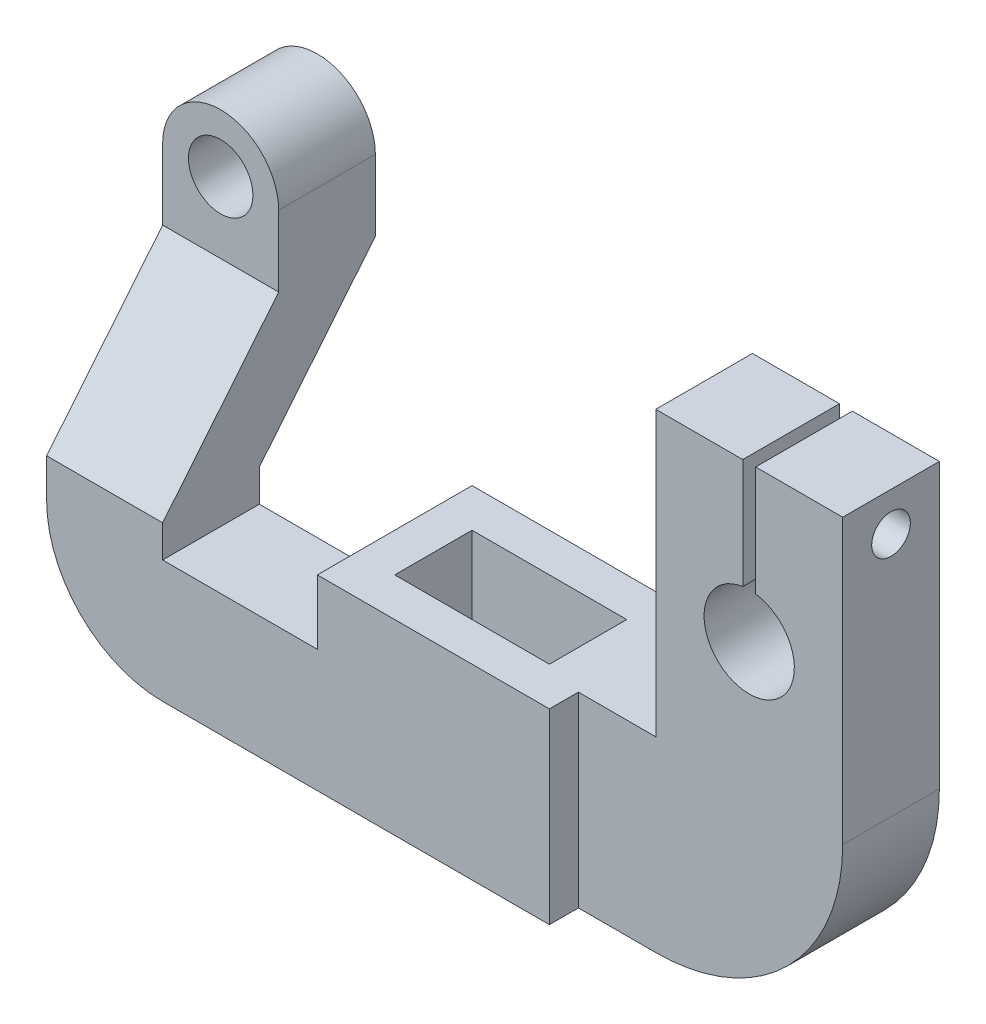
ISO-10303-21;
HEADER;
FILE_DESCRIPTION(('STEP AP214'),'2;1');
FILE_NAME('part.step','',(''),(''),'','','');
FILE_SCHEMA(('AUTOMOTIVE_DESIGN { 1 0 10303 214 1 1 1 1 }'));
ENDSEC;
DATA;
#1=APPLICATION_CONTEXT('core data for automotive mechanical design processes');
#2=APPLICATION_PROTOCOL_DEFINITION('international standard','automotive_design',2000,#1);
#3=PRODUCT_CONTEXT('',#1,'mechanical');
#4=PRODUCT('Part','Part','',(#3));
#5=PRODUCT_RELATED_PRODUCT_CATEGORY('part','',(#4));
#6=PRODUCT_DEFINITION_FORMATION('','',#4);
#7=PRODUCT_DEFINITION_CONTEXT('part definition',#1,'design');
#8=PRODUCT_DEFINITION('design','',#6,#7);
#9=PRODUCT_DEFINITION_SHAPE('','',#8);
#10=(LENGTH_UNIT() NAMED_UNIT(*) SI_UNIT(.MILLI.,.METRE.));
#11=(NAMED_UNIT(*) PLANE_ANGLE_UNIT() SI_UNIT($,.RADIAN.));
#12=(NAMED_UNIT(*) SI_UNIT($,.STERADIAN.) SOLID_ANGLE_UNIT());
#13=UNCERTAINTY_MEASURE_WITH_UNIT(LENGTH_MEASURE(1.E-05),#10,'distance_accuracy_value','');
#14=(GEOMETRIC_REPRESENTATION_CONTEXT(3) GLOBAL_UNCERTAINTY_ASSIGNED_CONTEXT((#13)) GLOBAL_UNIT_ASSIGNED_CONTEXT((#10,
#11,#12)) REPRESENTATION_CONTEXT('',''));
#15=CARTESIAN_POINT('',(0.,0.,0.));
#16=DIRECTION('',(0.,0.,1.));
#17=DIRECTION('',(1.,0.,0.));
#18=AXIS2_PLACEMENT_3D('',#15,#16,#17);
#19=CARTESIAN_POINT('',(0.,73.,-19.5));
#20=DIRECTION('',(0.,-1.,0.));
#21=DIRECTION('',(0.,0.,-1.));
#22=AXIS2_PLACEMENT_3D('',#19,#20,#21);
#23=PLANE('',#22);
#24=DIRECTION('',(1.,0.,0.));
#25=VECTOR('',#24,1.);
#26=CARTESIAN_POINT('',(0.,73.,-4.5));
#27=LINE('',#26,#25);
#28=CARTESIAN_POINT('',(72.,73.,-4.5));
#29=VERTEX_POINT('',#28);
#30=CARTESIAN_POINT('',(85.5,73.,-4.5));
#31=VERTEX_POINT('',#30);
#32=EDGE_CURVE('E374',#29,#31,#27,.T.);
#33=ORIENTED_EDGE('',*,*,#32,.T.);
#34=DIRECTION('',(0.,0.,1.));
#35=VECTOR('',#34,1.);
#36=CARTESIAN_POINT('',(85.5,73.,-19.5));
#37=LINE('',#36,#35);
#38=CARTESIAN_POINT('',(85.5,73.,-19.5));
#39=VERTEX_POINT('',#38);
#40=EDGE_CURVE('E269',#39,#31,#37,.T.);
#41=ORIENTED_EDGE('',*,*,#40,.F.);
#42=DIRECTION('',(1.,0.,0.));
#43=VECTOR('',#42,1.);
#44=CARTESIAN_POINT('',(0.,73.,-19.5));
#45=LINE('',#44,#43);
#46=CARTESIAN_POINT('',(72.,73.,-19.5));
#47=VERTEX_POINT('',#46);
#48=EDGE_CURVE('E356',#47,#39,#45,.T.);
#49=ORIENTED_EDGE('',*,*,#48,.F.);
#50=DIRECTION('',(0.,0.,1.));
#51=VECTOR('',#50,1.);
#52=CARTESIAN_POINT('',(72.,73.,-19.5));
#53=LINE('',#52,#51);
#54=EDGE_CURVE('E390',#47,#29,#53,.T.);
#55=ORIENTED_EDGE('',*,*,#54,.T.);
#56=EDGE_LOOP('',(#33,#41,#49,#55));
#57=FACE_BOUND('',#56,.T.);
#58=ADVANCED_FACE('F44',(#57),#23,.F.);
#59=CARTESIAN_POINT('',(60.,0.,-24.));
#60=DIRECTION('',(1.,0.,0.));
#61=DIRECTION('',(0.,0.,-1.));
#62=AXIS2_PLACEMENT_3D('',#59,#60,#61);
#63=PLANE('',#62);
#64=DIRECTION('',(0.,0.,1.));
#65=VECTOR('',#64,1.);
#66=CARTESIAN_POINT('',(60.,0.,-24.));
#67=LINE('',#66,#65);
#68=CARTESIAN_POINT('',(60.,0.,-4.5));
#69=VERTEX_POINT('',#68);
#70=CARTESIAN_POINT('',(60.,0.,0.));
#71=VERTEX_POINT('',#70);
#72=EDGE_CURVE('E424',#69,#71,#67,.T.);
#73=ORIENTED_EDGE('',*,*,#72,.F.);
#74=DIRECTION('',(0.,1.,0.));
#75=VECTOR('',#74,1.);
#76=CARTESIAN_POINT('',(60.,0.,-4.5));
#77=LINE('',#76,#75);
#78=CARTESIAN_POINT('',(60.,29.,-4.5));
#79=VERTEX_POINT('',#78);
#80=EDGE_CURVE('E348',#69,#79,#77,.T.);
#81=ORIENTED_EDGE('',*,*,#80,.T.);
#82=DIRECTION('',(0.,0.,1.));
#83=VECTOR('',#82,1.);
#84=CARTESIAN_POINT('',(60.,29.,-24.));
#85=LINE('',#84,#83);
#86=CARTESIAN_POINT('',(60.,29.,0.));
#87=VERTEX_POINT('',#86);
#88=EDGE_CURVE('E419',#79,#87,#85,.T.);
#89=ORIENTED_EDGE('',*,*,#88,.T.);
#90=DIRECTION('',(0.,1.,0.));
#91=VECTOR('',#90,1.);
#92=CARTESIAN_POINT('',(60.,0.,0.));
#93=LINE('',#92,#91);
#94=EDGE_CURVE('E400',#71,#87,#93,.T.);
#95=ORIENTED_EDGE('',*,*,#94,.F.);
#96=EDGE_LOOP('',(#73,#81,#89,#95));
#97=FACE_BOUND('',#96,.T.);
#98=ADVANCED_FACE('F484',(#97),#63,.T.);
#99=CARTESIAN_POINT('',(-18.,0.,-15.));
#100=DIRECTION('',(1.,0.,0.));
#101=DIRECTION('',(0.,0.,-1.));
#102=AXIS2_PLACEMENT_3D('',#99,#100,#101);
#103=PLANE('',#102);
#104=DIRECTION('',(0.,1.,0.));
#105=VECTOR('',#104,1.);
#106=CARTESIAN_POINT('',(-18.,0.,0.));
#107=LINE('',#106,#105);
#108=CARTESIAN_POINT('',(-18.,17.9999999999999,0.));
#109=VERTEX_POINT('',#108);
#110=CARTESIAN_POINT('',(-18.,24.,0.));
#111=VERTEX_POINT('',#110);
#112=EDGE_CURVE('E420',#109,#111,#107,.T.);
#113=ORIENTED_EDGE('',*,*,#112,.T.);
#114=DIRECTION('',(0.,0.773957299203321,-0.633237790257263));
#115=VECTOR('',#114,1.);
#116=CARTESIAN_POINT('',(-18.,46.,-18.));
#117=LINE('',#116,#115);
#118=CARTESIAN_POINT('',(-18.,46.,-18.));
#119=VERTEX_POINT('',#118);
#120=EDGE_CURVE('E329',#111,#119,#117,.T.);
#121=ORIENTED_EDGE('',*,*,#120,.T.);
#122=DIRECTION('',(0.,-1.,0.));
#123=VECTOR('',#122,1.);
#124=CARTESIAN_POINT('',(-18.,57.,-18.));
#125=LINE('',#124,#123);
#126=CARTESIAN_POINT('',(-18.,57.,-18.));
#127=VERTEX_POINT('',#126);
#128=EDGE_CURVE('E312',#127,#119,#125,.T.);
#129=ORIENTED_EDGE('',*,*,#128,.F.);
#130=DIRECTION('',(0.,0.,-1.));
#131=VECTOR('',#130,1.);
#132=CARTESIAN_POINT('',(-18.,57.,-18.));
#133=LINE('',#132,#131);
#134=CARTESIAN_POINT('',(-18.,57.,-33.));
#135=VERTEX_POINT('',#134);
#136=EDGE_CURVE('E318',#127,#135,#133,.T.);
#137=ORIENTED_EDGE('',*,*,#136,.T.);
#138=DIRECTION('',(0.,-1.,0.));
#139=VECTOR('',#138,1.);
#140=CARTESIAN_POINT('',(-18.,57.,-33.));
#141=LINE('',#140,#139);
#142=CARTESIAN_POINT('',(-18.,46.,-33.));
#143=VERTEX_POINT('',#142);
#144=EDGE_CURVE('E311',#135,#143,#141,.T.);
#145=ORIENTED_EDGE('',*,*,#144,.T.);
#146=DIRECTION('',(0.,-0.773957299203321,0.633237790257263));
#147=VECTOR('',#146,1.);
#148=CARTESIAN_POINT('',(-18.,46.,-33.));
#149=LINE('',#148,#147);
#150=CARTESIAN_POINT('',(-18.,24.,-15.));
#151=VERTEX_POINT('',#150);
#152=EDGE_CURVE('E331',#143,#151,#149,.T.);
#153=ORIENTED_EDGE('',*,*,#152,.T.);
#154=DIRECTION('',(0.,1.,0.));
#155=VECTOR('',#154,1.);
#156=CARTESIAN_POINT('',(-18.,0.,-15.));
#157=LINE('',#156,#155);
#158=CARTESIAN_POINT('',(-18.,17.9999999999999,-15.));
#159=VERTEX_POINT('',#158);
#160=EDGE_CURVE('E427',#159,#151,#157,.T.);
#161=ORIENTED_EDGE('',*,*,#160,.F.);
#162=DIRECTION('',(0.,0.,1.));
#163=VECTOR('',#162,1.);
#164=CARTESIAN_POINT('',(-18.,17.9999999999999,-15.));
#165=LINE('',#164,#163);
#166=EDGE_CURVE('E446',#159,#109,#165,.T.);
#167=ORIENTED_EDGE('',*,*,#166,.T.);
#168=EDGE_LOOP('',(#113,#121,#129,#137,#145,#153,#161,#167));
#169=FACE_BOUND('',#168,.T.);
#170=ADVANCED_FACE('F50',(#169),#103,.F.);
#171=CARTESIAN_POINT('',(0.,0.,-15.));
#172=DIRECTION('',(1.,0.,0.));
#173=DIRECTION('',(0.,1.,0.));
#174=AXIS2_PLACEMENT_3D('',#171,#172,#173);
#175=PLANE('',#174);
#176=DIRECTION('',(0.,1.,0.));
#177=VECTOR('',#176,1.);
#178=CARTESIAN_POINT('',(0.,0.,0.));
#179=LINE('',#178,#177);
#180=CARTESIAN_POINT('',(0.,19.,0.));
#181=VERTEX_POINT('',#180);
#182=CARTESIAN_POINT('',(0.,24.,0.));
#183=VERTEX_POINT('',#182);
#184=EDGE_CURVE('E462',#181,#183,#179,.T.);
#185=ORIENTED_EDGE('',*,*,#184,.F.);
#186=DIRECTION('',(0.,0.,1.));
#187=VECTOR('',#186,1.);
#188=CARTESIAN_POINT('',(0.,19.,-15.));
#189=LINE('',#188,#187);
#190=CARTESIAN_POINT('',(0.,19.,-15.));
#191=VERTEX_POINT('',#190);
#192=EDGE_CURVE('E11',#191,#181,#189,.T.);
#193=ORIENTED_EDGE('',*,*,#192,.F.);
#194=DIRECTION('',(0.,1.,0.));
#195=VECTOR('',#194,1.);
#196=CARTESIAN_POINT('',(0.,0.,-15.));
#197=LINE('',#196,#195);
#198=CARTESIAN_POINT('',(0.,24.,-15.));
#199=VERTEX_POINT('',#198);
#200=EDGE_CURVE('E441',#191,#199,#197,.T.);
#201=ORIENTED_EDGE('',*,*,#200,.T.);
#202=DIRECTION('',(0.,-0.773957299203321,0.633237790257263));
#203=VECTOR('',#202,1.);
#204=CARTESIAN_POINT('',(0.,46.,-33.));
#205=LINE('',#204,#203);
#206=CARTESIAN_POINT('',(0.,46.,-33.));
#207=VERTEX_POINT('',#206);
#208=EDGE_CURVE('E334',#207,#199,#205,.T.);
#209=ORIENTED_EDGE('',*,*,#208,.F.);
#210=DIRECTION('',(0.,1.,0.));
#211=VECTOR('',#210,1.);
#212=CARTESIAN_POINT('',(0.,46.,-33.));
#213=LINE('',#212,#211);
#214=CARTESIAN_POINT('',(0.,57.,-33.));
#215=VERTEX_POINT('',#214);
#216=EDGE_CURVE('E308',#207,#215,#213,.T.);
#217=ORIENTED_EDGE('',*,*,#216,.T.);
#218=DIRECTION('',(0.,0.,-1.));
#219=VECTOR('',#218,1.);
#220=CARTESIAN_POINT('',(0.,57.,-18.));
#221=LINE('',#220,#219);
#222=CARTESIAN_POINT('',(0.,57.,-18.));
#223=VERTEX_POINT('',#222);
#224=EDGE_CURVE('E330',#223,#215,#221,.T.);
#225=ORIENTED_EDGE('',*,*,#224,.F.);
#226=DIRECTION('',(0.,1.,0.));
#227=VECTOR('',#226,1.);
#228=CARTESIAN_POINT('',(0.,46.,-18.));
#229=LINE('',#228,#227);
#230=CARTESIAN_POINT('',(0.,46.,-18.));
#231=VERTEX_POINT('',#230);
#232=EDGE_CURVE('E310',#231,#223,#229,.T.);
#233=ORIENTED_EDGE('',*,*,#232,.F.);
#234=DIRECTION('',(0.,0.773957299203321,-0.633237790257263));
#235=VECTOR('',#234,1.);
#236=CARTESIAN_POINT('',(0.,46.,-18.));
#237=LINE('',#236,#235);
#238=EDGE_CURVE('E332',#183,#231,#237,.T.);
#239=ORIENTED_EDGE('',*,*,#238,.F.);
#240=EDGE_LOOP('',(#185,#193,#201,#209,#217,#225,#233,#239));
#241=FACE_BOUND('',#240,.T.);
#242=ADVANCED_FACE('F507',(#241),#175,.T.);
#243=CARTESIAN_POINT('',(0.,19.,-15.));
#244=DIRECTION('',(0.,1.,0.));
#245=DIRECTION('',(-1.,0.,0.));
#246=AXIS2_PLACEMENT_3D('',#243,#244,#245);
#247=PLANE('',#246);
#248=DIRECTION('',(-1.,0.,0.));
#249=VECTOR('',#248,1.);
#250=CARTESIAN_POINT('',(0.,19.,0.));
#251=LINE('',#250,#249);
#252=CARTESIAN_POINT('',(24.,19.,0.));
#253=VERTEX_POINT('',#252);
#254=EDGE_CURVE('E456',#253,#181,#251,.T.);
#255=ORIENTED_EDGE('',*,*,#254,.F.);
#256=DIRECTION('',(0.,0.,1.));
#257=VECTOR('',#256,1.);
#258=CARTESIAN_POINT('',(24.,19.,-15.));
#259=LINE('',#258,#257);
#260=CARTESIAN_POINT('',(24.,19.,-15.));
#261=VERTEX_POINT('',#260);
#262=EDGE_CURVE('E53',#261,#253,#259,.T.);
#263=ORIENTED_EDGE('',*,*,#262,.F.);
#264=DIRECTION('',(-1.,0.,0.));
#265=VECTOR('',#264,1.);
#266=CARTESIAN_POINT('',(0.,19.,-15.));
#267=LINE('',#266,#265);
#268=EDGE_CURVE('E442',#261,#191,#267,.T.);
#269=ORIENTED_EDGE('',*,*,#268,.T.);
#270=ORIENTED_EDGE('',*,*,#192,.T.);
#271=EDGE_LOOP('',(#255,#263,#269,#270));
#272=FACE_BOUND('',#271,.T.);
#273=ADVANCED_FACE('F496',(#272),#247,.T.);
#274=CARTESIAN_POINT('',(0.,0.,-15.));
#275=DIRECTION('',(0.,-1.,0.));
#276=DIRECTION('',(0.,0.,-1.));
#277=AXIS2_PLACEMENT_3D('',#274,#275,#276);
#278=PLANE('',#277);
#279=DIRECTION('',(0.,0.,1.));
#280=VECTOR('',#279,1.);
#281=CARTESIAN_POINT('',(30.,0.,-18.));
#282=LINE('',#281,#280);
#283=CARTESIAN_POINT('',(30.,0.,-18.));
#284=VERTEX_POINT('',#283);
#285=CARTESIAN_POINT('',(30.,0.,-6.00000000000001));
#286=VERTEX_POINT('',#285);
#287=EDGE_CURVE('E272',#284,#286,#282,.T.);
#288=ORIENTED_EDGE('',*,*,#287,.T.);
#289=DIRECTION('',(1.,0.,0.));
#290=VECTOR('',#289,1.);
#291=CARTESIAN_POINT('',(30.,0.,-6.00000000000001));
#292=LINE('',#291,#290);
#293=CARTESIAN_POINT('',(54.,0.,-6.00000000000001));
#294=VERTEX_POINT('',#293);
#295=EDGE_CURVE('E277',#286,#294,#292,.T.);
#296=ORIENTED_EDGE('',*,*,#295,.T.);
#297=DIRECTION('',(0.,0.,-1.));
#298=VECTOR('',#297,1.);
#299=CARTESIAN_POINT('',(54.,0.,-18.));
#300=LINE('',#299,#298);
#301=CARTESIAN_POINT('',(54.,0.,-18.));
#302=VERTEX_POINT('',#301);
#303=EDGE_CURVE('E70',#294,#302,#300,.T.);
#304=ORIENTED_EDGE('',*,*,#303,.T.);
#305=DIRECTION('',(-1.,0.,0.));
#306=VECTOR('',#305,1.);
#307=CARTESIAN_POINT('',(30.,0.,-18.));
#308=LINE('',#307,#306);
#309=EDGE_CURVE('E282',#302,#284,#308,.T.);
#310=ORIENTED_EDGE('',*,*,#309,.T.);
#311=EDGE_LOOP('',(#288,#296,#304,#310));
#312=FACE_BOUND('',#311,.T.);
#313=DIRECTION('',(1.,0.,0.));
#314=VECTOR('',#313,1.);
#315=CARTESIAN_POINT('',(0.,0.,0.));
#316=LINE('',#315,#314);
#317=CARTESIAN_POINT('',(0.,0.,0.));
#318=VERTEX_POINT('',#317);
#319=EDGE_CURVE('E455',#318,#71,#316,.T.);
#320=ORIENTED_EDGE('',*,*,#319,.F.);
#321=DIRECTION('',(0.,0.,1.));
#322=VECTOR('',#321,1.);
#323=CARTESIAN_POINT('',(0.,0.,-15.));
#324=LINE('',#323,#322);
#325=CARTESIAN_POINT('',(0.,0.,-15.));
#326=VERTEX_POINT('',#325);
#327=EDGE_CURVE('E469',#326,#318,#324,.T.);
#328=ORIENTED_EDGE('',*,*,#327,.F.);
#329=DIRECTION('',(1.,0.,0.));
#330=VECTOR('',#329,1.);
#331=CARTESIAN_POINT('',(0.,0.,-15.));
#332=LINE('',#331,#330);
#333=CARTESIAN_POINT('',(24.,0.,-15.));
#334=VERTEX_POINT('',#333);
#335=EDGE_CURVE('E436',#326,#334,#332,.T.);
#336=ORIENTED_EDGE('',*,*,#335,.T.);
#337=DIRECTION('',(0.,0.,1.));
#338=VECTOR('',#337,1.);
#339=CARTESIAN_POINT('',(24.,0.,-24.));
#340=LINE('',#339,#338);
#341=CARTESIAN_POINT('',(24.,0.,-24.));
#342=VERTEX_POINT('',#341);
#343=EDGE_CURVE('E422',#342,#334,#340,.T.);
#344=ORIENTED_EDGE('',*,*,#343,.F.);
#345=DIRECTION('',(1.,0.,0.));
#346=VECTOR('',#345,1.);
#347=CARTESIAN_POINT('',(0.,0.,-24.));
#348=LINE('',#347,#346);
#349=CARTESIAN_POINT('',(60.,0.,-24.));
#350=VERTEX_POINT('',#349);
#351=EDGE_CURVE('E401',#342,#350,#348,.T.);
#352=ORIENTED_EDGE('',*,*,#351,.T.);
#353=CARTESIAN_POINT('',(60.,0.,-19.5));
#354=VERTEX_POINT('',#353);
#355=EDGE_CURVE('E423',#350,#354,#67,.T.);
#356=ORIENTED_EDGE('',*,*,#355,.T.);
#357=DIRECTION('',(1.,0.,0.));
#358=VECTOR('',#357,1.);
#359=CARTESIAN_POINT('',(0.,0.,-19.5));
#360=LINE('',#359,#358);
#361=CARTESIAN_POINT('',(72.,0.,-19.5));
#362=VERTEX_POINT('',#361);
#363=EDGE_CURVE('E347',#354,#362,#360,.T.);
#364=ORIENTED_EDGE('',*,*,#363,.T.);
#365=DIRECTION('',(0.,0.,1.));
#366=VECTOR('',#365,1.);
#367=CARTESIAN_POINT('',(72.,0.,-19.5));
#368=LINE('',#367,#366);
#369=CARTESIAN_POINT('',(72.,0.,-4.5));
#370=VERTEX_POINT('',#369);
#371=EDGE_CURVE('E364',#362,#370,#368,.T.);
#372=ORIENTED_EDGE('',*,*,#371,.T.);
#373=DIRECTION('',(1.,0.,0.));
#374=VECTOR('',#373,1.);
#375=CARTESIAN_POINT('',(0.,0.,-4.5));
#376=LINE('',#375,#374);
#377=EDGE_CURVE('E343',#69,#370,#376,.T.);
#378=ORIENTED_EDGE('',*,*,#377,.F.);
#379=ORIENTED_EDGE('',*,*,#72,.T.);
#380=EDGE_LOOP('',(#320,#328,#336,#344,#352,#356,#364,#372,#378,#379));
#381=FACE_BOUND('',#380,.T.);
#382=ADVANCED_FACE('F481',(#312,#381),#278,.T.);
#383=CARTESIAN_POINT('',(0.,18.,-15.));
#384=DIRECTION('',(0.,0.,1.));
#385=DIRECTION('',(1.,0.,0.));
#386=AXIS2_PLACEMENT_3D('',#383,#384,#385);
#387=CYLINDRICAL_SURFACE('',#386,18.);
#388=CARTESIAN_POINT('',(0.,18.,0.));
#389=DIRECTION('',(0.,0.,1.));
#390=DIRECTION('',(1.,0.,0.));
#391=AXIS2_PLACEMENT_3D('',#388,#389,#390);
#392=CIRCLE('',#391,18.);
#393=EDGE_CURVE('E452',#109,#318,#392,.T.);
#394=ORIENTED_EDGE('',*,*,#393,.F.);
#395=ORIENTED_EDGE('',*,*,#166,.F.);
#396=CARTESIAN_POINT('',(0.,18.,-15.));
#397=DIRECTION('',(0.,0.,1.));
#398=DIRECTION('',(1.,0.,0.));
#399=AXIS2_PLACEMENT_3D('',#396,#397,#398);
#400=CIRCLE('',#399,18.);
#401=EDGE_CURVE('E435',#159,#326,#400,.T.);
#402=ORIENTED_EDGE('',*,*,#401,.T.);
#403=ORIENTED_EDGE('',*,*,#327,.T.);
#404=EDGE_LOOP('',(#394,#395,#402,#403));
#405=FACE_BOUND('',#404,.T.);
#406=ADVANCED_FACE('F480',(#405),#387,.T.);
#407=CARTESIAN_POINT('',(0.,0.,-15.));
#408=DIRECTION('',(0.,0.,1.));
#409=DIRECTION('',(1.,0.,0.));
#410=AXIS2_PLACEMENT_3D('',#407,#408,#409);
#411=PLANE('',#410);
#412=ORIENTED_EDGE('',*,*,#160,.T.);
#413=DIRECTION('',(-1.,0.,0.));
#414=VECTOR('',#413,1.);
#415=CARTESIAN_POINT('',(0.,24.,-15.));
#416=LINE('',#415,#414);
#417=EDGE_CURVE('E449',#199,#151,#416,.T.);
#418=ORIENTED_EDGE('',*,*,#417,.F.);
#419=ORIENTED_EDGE('',*,*,#200,.F.);
#420=ORIENTED_EDGE('',*,*,#268,.F.);
#421=DIRECTION('',(0.,-1.,0.));
#422=VECTOR('',#421,1.);
#423=CARTESIAN_POINT('',(24.,0.,-15.));
#424=LINE('',#423,#422);
#425=EDGE_CURVE('E438',#261,#334,#424,.T.);
#426=ORIENTED_EDGE('',*,*,#425,.T.);
#427=ORIENTED_EDGE('',*,*,#335,.F.);
#428=ORIENTED_EDGE('',*,*,#401,.F.);
#429=EDGE_LOOP('',(#412,#418,#419,#420,#426,#427,#428));
#430=FACE_BOUND('',#429,.T.);
#431=ADVANCED_FACE('F504',(#430),#411,.F.);
#432=CARTESIAN_POINT('',(0.,0.,0.));
#433=DIRECTION('',(0.,0.,1.));
#434=DIRECTION('',(1.,0.,0.));
#435=AXIS2_PLACEMENT_3D('',#432,#433,#434);
#436=PLANE('',#435);
#437=ORIENTED_EDGE('',*,*,#112,.F.);
#438=ORIENTED_EDGE('',*,*,#393,.T.);
#439=ORIENTED_EDGE('',*,*,#319,.T.);
#440=ORIENTED_EDGE('',*,*,#94,.T.);
#441=DIRECTION('',(-1.,0.,0.));
#442=VECTOR('',#441,1.);
#443=CARTESIAN_POINT('',(0.,29.,0.));
#444=LINE('',#443,#442);
#445=CARTESIAN_POINT('',(24.,29.,0.));
#446=VERTEX_POINT('',#445);
#447=EDGE_CURVE('E387',#87,#446,#444,.T.);
#448=ORIENTED_EDGE('',*,*,#447,.T.);
#449=DIRECTION('',(0.,-1.,0.));
#450=VECTOR('',#449,1.);
#451=CARTESIAN_POINT('',(24.,0.,0.));
#452=LINE('',#451,#450);
#453=EDGE_CURVE('E412',#446,#253,#452,.T.);
#454=ORIENTED_EDGE('',*,*,#453,.T.);
#455=ORIENTED_EDGE('',*,*,#254,.T.);
#456=ORIENTED_EDGE('',*,*,#184,.T.);
#457=DIRECTION('',(-1.,0.,0.));
#458=VECTOR('',#457,1.);
#459=CARTESIAN_POINT('',(0.,24.,0.));
#460=LINE('',#459,#458);
#461=EDGE_CURVE('E433',#183,#111,#460,.T.);
#462=ORIENTED_EDGE('',*,*,#461,.T.);
#463=EDGE_LOOP('',(#437,#438,#439,#440,#448,#454,#455,#456,#462));
#464=FACE_BOUND('',#463,.T.);
#465=ADVANCED_FACE('F478',(#464),#436,.T.);
#466=CARTESIAN_POINT('',(24.,0.,-24.));
#467=DIRECTION('',(-1.,0.,0.));
#468=DIRECTION('',(0.,0.,1.));
#469=AXIS2_PLACEMENT_3D('',#466,#467,#468);
#470=PLANE('',#469);
#471=ORIENTED_EDGE('',*,*,#425,.F.);
#472=ORIENTED_EDGE('',*,*,#262,.T.);
#473=ORIENTED_EDGE('',*,*,#453,.F.);
#474=DIRECTION('',(0.,0.,1.));
#475=VECTOR('',#474,1.);
#476=CARTESIAN_POINT('',(24.,29.,-24.));
#477=LINE('',#476,#475);
#478=CARTESIAN_POINT('',(24.,29.,-24.));
#479=VERTEX_POINT('',#478);
#480=EDGE_CURVE('E406',#479,#446,#477,.T.);
#481=ORIENTED_EDGE('',*,*,#480,.F.);
#482=DIRECTION('',(0.,-1.,0.));
#483=VECTOR('',#482,1.);
#484=CARTESIAN_POINT('',(24.,0.,-24.));
#485=LINE('',#484,#483);
#486=EDGE_CURVE('E398',#479,#342,#485,.T.);
#487=ORIENTED_EDGE('',*,*,#486,.T.);
#488=ORIENTED_EDGE('',*,*,#343,.T.);
#489=EDGE_LOOP('',(#471,#472,#473,#481,#487,#488));
#490=FACE_BOUND('',#489,.T.);
#491=ADVANCED_FACE('F494',(#490),#470,.T.);
#492=CARTESIAN_POINT('',(0.,29.,-24.));
#493=DIRECTION('',(0.,1.,0.));
#494=DIRECTION('',(-1.,0.,0.));
#495=AXIS2_PLACEMENT_3D('',#492,#493,#494);
#496=PLANE('',#495);
#497=DIRECTION('',(0.,0.,1.));
#498=VECTOR('',#497,1.);
#499=CARTESIAN_POINT('',(30.,29.,-18.));
#500=LINE('',#499,#498);
#501=CARTESIAN_POINT('',(30.,29.,-18.));
#502=VERTEX_POINT('',#501);
#503=CARTESIAN_POINT('',(30.,29.,-6.));
#504=VERTEX_POINT('',#503);
#505=EDGE_CURVE('E267',#502,#504,#500,.T.);
#506=ORIENTED_EDGE('',*,*,#505,.F.);
#507=DIRECTION('',(-1.,0.,0.));
#508=VECTOR('',#507,1.);
#509=CARTESIAN_POINT('',(30.,29.,-18.));
#510=LINE('',#509,#508);
#511=CARTESIAN_POINT('',(54.,29.,-18.));
#512=VERTEX_POINT('',#511);
#513=EDGE_CURVE('E280',#512,#502,#510,.T.);
#514=ORIENTED_EDGE('',*,*,#513,.F.);
#515=DIRECTION('',(0.,0.,-1.));
#516=VECTOR('',#515,1.);
#517=CARTESIAN_POINT('',(54.,29.,-18.));
#518=LINE('',#517,#516);
#519=CARTESIAN_POINT('',(54.,29.,-6.00000000000001));
#520=VERTEX_POINT('',#519);
#521=EDGE_CURVE('E288',#520,#512,#518,.T.);
#522=ORIENTED_EDGE('',*,*,#521,.F.);
#523=DIRECTION('',(1.,0.,0.));
#524=VECTOR('',#523,1.);
#525=CARTESIAN_POINT('',(30.,29.,-6.00000000000001));
#526=LINE('',#525,#524);
#527=EDGE_CURVE('E286',#504,#520,#526,.T.);
#528=ORIENTED_EDGE('',*,*,#527,.F.);
#529=EDGE_LOOP('',(#506,#514,#522,#528));
#530=FACE_BOUND('',#529,.T.);
#531=ORIENTED_EDGE('',*,*,#447,.F.);
#532=ORIENTED_EDGE('',*,*,#88,.F.);
#533=DIRECTION('',(1.,0.,0.));
#534=VECTOR('',#533,1.);
#535=CARTESIAN_POINT('',(0.,29.,-4.5));
#536=LINE('',#535,#534);
#537=CARTESIAN_POINT('',(72.,29.,-4.5));
#538=VERTEX_POINT('',#537);
#539=EDGE_CURVE('E379',#79,#538,#536,.T.);
#540=ORIENTED_EDGE('',*,*,#539,.T.);
#541=DIRECTION('',(0.,0.,1.));
#542=VECTOR('',#541,1.);
#543=CARTESIAN_POINT('',(72.,29.,-19.5));
#544=LINE('',#543,#542);
#545=CARTESIAN_POINT('',(72.,29.,-19.5));
#546=VERTEX_POINT('',#545);
#547=EDGE_CURVE('E382',#546,#538,#544,.T.);
#548=ORIENTED_EDGE('',*,*,#547,.F.);
#549=DIRECTION('',(1.,0.,0.));
#550=VECTOR('',#549,1.);
#551=CARTESIAN_POINT('',(0.,29.,-19.5));
#552=LINE('',#551,#550);
#553=CARTESIAN_POINT('',(60.,29.,-19.5));
#554=VERTEX_POINT('',#553);
#555=EDGE_CURVE('E360',#554,#546,#552,.T.);
#556=ORIENTED_EDGE('',*,*,#555,.F.);
#557=CARTESIAN_POINT('',(60.,29.,-24.));
#558=VERTEX_POINT('',#557);
#559=EDGE_CURVE('E417',#558,#554,#85,.T.);
#560=ORIENTED_EDGE('',*,*,#559,.F.);
#561=DIRECTION('',(-1.,0.,0.));
#562=VECTOR('',#561,1.);
#563=CARTESIAN_POINT('',(0.,29.,-24.));
#564=LINE('',#563,#562);
#565=EDGE_CURVE('E396',#558,#479,#564,.T.);
#566=ORIENTED_EDGE('',*,*,#565,.T.);
#567=ORIENTED_EDGE('',*,*,#480,.T.);
#568=EDGE_LOOP('',(#531,#532,#540,#548,#556,#560,#566,#567));
#569=FACE_BOUND('',#568,.T.);
#570=ADVANCED_FACE('F491',(#530,#569),#496,.T.);
#571=DIRECTION('',(0.,1.,0.));
#572=VECTOR('',#571,1.);
#573=CARTESIAN_POINT('',(60.,0.,-19.5));
#574=LINE('',#573,#572);
#575=EDGE_CURVE('E362',#354,#554,#574,.T.);
#576=ORIENTED_EDGE('',*,*,#575,.F.);
#577=ORIENTED_EDGE('',*,*,#355,.F.);
#578=DIRECTION('',(0.,1.,0.));
#579=VECTOR('',#578,1.);
#580=CARTESIAN_POINT('',(60.,0.,-24.));
#581=LINE('',#580,#579);
#582=EDGE_CURVE('E407',#350,#558,#581,.T.);
#583=ORIENTED_EDGE('',*,*,#582,.T.);
#584=ORIENTED_EDGE('',*,*,#559,.T.);
#585=EDGE_LOOP('',(#576,#577,#583,#584));
#586=FACE_BOUND('',#585,.T.);
#587=ADVANCED_FACE('F531',(#586),#63,.T.);
#588=CARTESIAN_POINT('',(0.,0.,-24.));
#589=DIRECTION('',(0.,0.,1.));
#590=DIRECTION('',(1.,0.,0.));
#591=AXIS2_PLACEMENT_3D('',#588,#589,#590);
#592=PLANE('',#591);
#593=ORIENTED_EDGE('',*,*,#565,.F.);
#594=ORIENTED_EDGE('',*,*,#582,.F.);
#595=ORIENTED_EDGE('',*,*,#351,.F.);
#596=ORIENTED_EDGE('',*,*,#486,.F.);
#597=EDGE_LOOP('',(#593,#594,#595,#596));
#598=FACE_BOUND('',#597,.T.);
#599=ADVANCED_FACE('F526',(#598),#592,.F.);
#600=CARTESIAN_POINT('',(72.,0.,-19.5));
#601=DIRECTION('',(1.,0.,0.));
#602=DIRECTION('',(0.,0.,-1.));
#603=AXIS2_PLACEMENT_3D('',#600,#601,#602);
#604=PLANE('',#603);
#605=CARTESIAN_POINT('',(72.,67.,-12.));
#606=DIRECTION('',(-1.,0.,0.));
#607=DIRECTION('',(0.,0.,1.));
#608=AXIS2_PLACEMENT_3D('',#605,#606,#607);
#609=CIRCLE('',#608,3.);
#610=CARTESIAN_POINT('',(72.,67.,-9.));
#611=VERTEX_POINT('',#610);
#612=EDGE_CURVE('E636',#611,#611,#609,.T.);
#613=ORIENTED_EDGE('',*,*,#612,.F.);
#614=EDGE_LOOP('',(#613));
#615=FACE_BOUND('',#614,.T.);
#616=DIRECTION('',(0.,1.,0.));
#617=VECTOR('',#616,1.);
#618=CARTESIAN_POINT('',(72.,0.,-4.5));
#619=LINE('',#618,#617);
#620=EDGE_CURVE('E378',#538,#29,#619,.T.);
#621=ORIENTED_EDGE('',*,*,#620,.T.);
#622=ORIENTED_EDGE('',*,*,#54,.F.);
#623=DIRECTION('',(0.,1.,0.));
#624=VECTOR('',#623,1.);
#625=CARTESIAN_POINT('',(72.,0.,-19.5));
#626=LINE('',#625,#624);
#627=EDGE_CURVE('E359',#546,#47,#626,.T.);
#628=ORIENTED_EDGE('',*,*,#627,.F.);
#629=ORIENTED_EDGE('',*,*,#547,.T.);
#630=EDGE_LOOP('',(#621,#622,#628,#629));
#631=FACE_BOUND('',#630,.T.);
#632=ADVANCED_FACE('F547',(#615,#631),#604,.F.);
#633=CARTESIAN_POINT('',(87.5,73.,-19.5));
#634=VERTEX_POINT('',#633);
#635=CARTESIAN_POINT('',(101.,73.,-19.5));
#636=VERTEX_POINT('',#635);
#637=EDGE_CURVE('E353',#634,#636,#45,.T.);
#638=ORIENTED_EDGE('',*,*,#637,.F.);
#639=DIRECTION('',(0.,0.,1.));
#640=VECTOR('',#639,1.);
#641=CARTESIAN_POINT('',(87.5,73.,-19.5));
#642=LINE('',#641,#640);
#643=CARTESIAN_POINT('',(87.5,73.,-4.5));
#644=VERTEX_POINT('',#643);
#645=EDGE_CURVE('E245',#634,#644,#642,.T.);
#646=ORIENTED_EDGE('',*,*,#645,.T.);
#647=CARTESIAN_POINT('',(101.,73.,-4.5));
#648=VERTEX_POINT('',#647);
#649=EDGE_CURVE('E372',#644,#648,#27,.T.);
#650=ORIENTED_EDGE('',*,*,#649,.T.);
#651=DIRECTION('',(0.,0.,1.));
#652=VECTOR('',#651,1.);
#653=CARTESIAN_POINT('',(101.,73.,-19.5));
#654=LINE('',#653,#652);
#655=EDGE_CURVE('E388',#636,#648,#654,.T.);
#656=ORIENTED_EDGE('',*,*,#655,.F.);
#657=EDGE_LOOP('',(#638,#646,#650,#656));
#658=FACE_BOUND('',#657,.T.);
#659=ADVANCED_FACE('F559',(#658),#23,.F.);
#660=CARTESIAN_POINT('',(101.,0.,-19.5));
#661=DIRECTION('',(-1.,0.,0.));
#662=DIRECTION('',(0.,0.,1.));
#663=AXIS2_PLACEMENT_3D('',#660,#661,#662);
#664=PLANE('',#663);
#665=CARTESIAN_POINT('',(101.,67.,-12.));
#666=DIRECTION('',(-1.,0.,0.));
#667=DIRECTION('',(0.,0.,1.));
#668=AXIS2_PLACEMENT_3D('',#665,#666,#667);
#669=CIRCLE('',#668,3.);
#670=CARTESIAN_POINT('',(101.,67.,-9.));
#671=VERTEX_POINT('',#670);
#672=EDGE_CURVE('E645',#671,#671,#669,.T.);
#673=ORIENTED_EDGE('',*,*,#672,.T.);
#674=EDGE_LOOP('',(#673));
#675=FACE_BOUND('',#674,.T.);
#676=DIRECTION('',(0.,-1.,0.));
#677=VECTOR('',#676,1.);
#678=CARTESIAN_POINT('',(101.,0.,-4.5));
#679=LINE('',#678,#677);
#680=CARTESIAN_POINT('',(101.,29.,-4.5));
#681=VERTEX_POINT('',#680);
#682=EDGE_CURVE('E371',#648,#681,#679,.T.);
#683=ORIENTED_EDGE('',*,*,#682,.T.);
#684=DIRECTION('',(0.,0.,1.));
#685=VECTOR('',#684,1.);
#686=CARTESIAN_POINT('',(101.,29.,-19.5));
#687=LINE('',#686,#685);
#688=CARTESIAN_POINT('',(101.,29.,-19.5));
#689=VERTEX_POINT('',#688);
#690=EDGE_CURVE('E395',#689,#681,#687,.T.);
#691=ORIENTED_EDGE('',*,*,#690,.F.);
#692=DIRECTION('',(0.,-1.,0.));
#693=VECTOR('',#692,1.);
#694=CARTESIAN_POINT('',(101.,0.,-19.5));
#695=LINE('',#694,#693);
#696=EDGE_CURVE('E355',#636,#689,#695,.T.);
#697=ORIENTED_EDGE('',*,*,#696,.F.);
#698=ORIENTED_EDGE('',*,*,#655,.T.);
#699=EDGE_LOOP('',(#683,#691,#697,#698));
#700=FACE_BOUND('',#699,.T.);
#701=ADVANCED_FACE('F561',(#675,#700),#664,.F.);
#702=CARTESIAN_POINT('',(72.,29.,-19.5));
#703=DIRECTION('',(0.,0.,1.));
#704=DIRECTION('',(1.,0.,0.));
#705=AXIS2_PLACEMENT_3D('',#702,#703,#704);
#706=CYLINDRICAL_SURFACE('',#705,29.);
#707=CARTESIAN_POINT('',(72.,29.,-4.5));
#708=DIRECTION('',(0.,0.,1.));
#709=DIRECTION('',(1.,0.,0.));
#710=AXIS2_PLACEMENT_3D('',#707,#708,#709);
#711=CIRCLE('',#710,29.);
#712=EDGE_CURVE('E366',#370,#681,#711,.T.);
#713=ORIENTED_EDGE('',*,*,#712,.F.);
#714=ORIENTED_EDGE('',*,*,#371,.F.);
#715=CARTESIAN_POINT('',(72.,29.,-19.5));
#716=DIRECTION('',(0.,0.,1.));
#717=DIRECTION('',(1.,0.,0.));
#718=AXIS2_PLACEMENT_3D('',#715,#716,#717);
#719=CIRCLE('',#718,29.);
#720=EDGE_CURVE('E349',#362,#689,#719,.T.);
#721=ORIENTED_EDGE('',*,*,#720,.T.);
#722=ORIENTED_EDGE('',*,*,#690,.T.);
#723=EDGE_LOOP('',(#713,#714,#721,#722));
#724=FACE_BOUND('',#723,.T.);
#725=ADVANCED_FACE('F538',(#724),#706,.T.);
#726=CARTESIAN_POINT('',(0.,0.,-19.5));
#727=DIRECTION('',(0.,0.,1.));
#728=DIRECTION('',(1.,0.,0.));
#729=AXIS2_PLACEMENT_3D('',#726,#727,#728);
#730=PLANE('',#729);
#731=ORIENTED_EDGE('',*,*,#48,.T.);
#732=DIRECTION('',(0.,-1.,0.));
#733=VECTOR('',#732,1.);
#734=CARTESIAN_POINT('',(85.5,55.9282032302755,-19.5));
#735=LINE('',#734,#733);
#736=CARTESIAN_POINT('',(85.5,55.9282032302755,-19.5));
#737=VERTEX_POINT('',#736);
#738=EDGE_CURVE('E241',#39,#737,#735,.T.);
#739=ORIENTED_EDGE('',*,*,#738,.T.);
#740=CARTESIAN_POINT('',(86.5,49.,-19.5));
#741=DIRECTION('',(0.,0.,1.));
#742=DIRECTION('',(1.,0.,0.));
#743=AXIS2_PLACEMENT_3D('',#740,#741,#742);
#744=CIRCLE('',#743,7.);
#745=CARTESIAN_POINT('',(87.5,55.9282032302755,-19.5));
#746=VERTEX_POINT('',#745);
#747=EDGE_CURVE('E239',#737,#746,#744,.T.);
#748=ORIENTED_EDGE('',*,*,#747,.T.);
#749=DIRECTION('',(0.,1.,0.));
#750=VECTOR('',#749,1.);
#751=CARTESIAN_POINT('',(87.5,55.9282032302755,-19.5));
#752=LINE('',#751,#750);
#753=EDGE_CURVE('E247',#746,#634,#752,.T.);
#754=ORIENTED_EDGE('',*,*,#753,.T.);
#755=ORIENTED_EDGE('',*,*,#637,.T.);
#756=ORIENTED_EDGE('',*,*,#696,.T.);
#757=ORIENTED_EDGE('',*,*,#720,.F.);
#758=ORIENTED_EDGE('',*,*,#363,.F.);
#759=ORIENTED_EDGE('',*,*,#575,.T.);
#760=ORIENTED_EDGE('',*,*,#555,.T.);
#761=ORIENTED_EDGE('',*,*,#627,.T.);
#762=EDGE_LOOP('',(#731,#739,#748,#754,#755,#756,#757,#758,#759,#760,#761));
#763=FACE_BOUND('',#762,.T.);
#764=ADVANCED_FACE('F255',(#763),#730,.F.);
#765=CARTESIAN_POINT('',(0.,0.,-4.5));
#766=DIRECTION('',(0.,0.,1.));
#767=DIRECTION('',(1.,0.,0.));
#768=AXIS2_PLACEMENT_3D('',#765,#766,#767);
#769=PLANE('',#768);
#770=DIRECTION('',(0.,-1.,0.));
#771=VECTOR('',#770,1.);
#772=CARTESIAN_POINT('',(85.5,55.9282032302755,-4.5));
#773=LINE('',#772,#771);
#774=CARTESIAN_POINT('',(85.5,55.9282032302755,-4.5));
#775=VERTEX_POINT('',#774);
#776=EDGE_CURVE('E254',#31,#775,#773,.T.);
#777=ORIENTED_EDGE('',*,*,#776,.F.);
#778=ORIENTED_EDGE('',*,*,#32,.F.);
#779=ORIENTED_EDGE('',*,*,#620,.F.);
#780=ORIENTED_EDGE('',*,*,#539,.F.);
#781=ORIENTED_EDGE('',*,*,#80,.F.);
#782=ORIENTED_EDGE('',*,*,#377,.T.);
#783=ORIENTED_EDGE('',*,*,#712,.T.);
#784=ORIENTED_EDGE('',*,*,#682,.F.);
#785=ORIENTED_EDGE('',*,*,#649,.F.);
#786=DIRECTION('',(0.,1.,0.));
#787=VECTOR('',#786,1.);
#788=CARTESIAN_POINT('',(87.5,55.9282032302755,-4.5));
#789=LINE('',#788,#787);
#790=CARTESIAN_POINT('',(87.5,55.9282032302755,-4.5));
#791=VERTEX_POINT('',#790);
#792=EDGE_CURVE('E256',#791,#644,#789,.T.);
#793=ORIENTED_EDGE('',*,*,#792,.F.);
#794=CARTESIAN_POINT('',(86.5,49.,-4.5));
#795=DIRECTION('',(0.,0.,1.));
#796=DIRECTION('',(1.,0.,0.));
#797=AXIS2_PLACEMENT_3D('',#794,#795,#796);
#798=CIRCLE('',#797,7.);
#799=EDGE_CURVE('E64',#775,#791,#798,.T.);
#800=ORIENTED_EDGE('',*,*,#799,.F.);
#801=EDGE_LOOP('',(#777,#778,#779,#780,#781,#782,#783,#784,#785,#793,#800));
#802=FACE_BOUND('',#801,.T.);
#803=ADVANCED_FACE('F543',(#802),#769,.T.);
#804=CARTESIAN_POINT('',(0.,46.,-33.));
#805=DIRECTION('',(0.,-0.633237790257263,-0.773957299203321));
#806=DIRECTION('',(0.,0.773957299203321,-0.633237790257263));
#807=AXIS2_PLACEMENT_3D('',#804,#805,#806);
#808=PLANE('',#807);
#809=ORIENTED_EDGE('',*,*,#152,.F.);
#810=DIRECTION('',(-1.,0.,0.));
#811=VECTOR('',#810,1.);
#812=CARTESIAN_POINT('',(0.,46.,-33.));
#813=LINE('',#812,#811);
#814=EDGE_CURVE('E341',#207,#143,#813,.T.);
#815=ORIENTED_EDGE('',*,*,#814,.F.);
#816=ORIENTED_EDGE('',*,*,#208,.T.);
#817=ORIENTED_EDGE('',*,*,#417,.T.);
#818=EDGE_LOOP('',(#809,#815,#816,#817));
#819=FACE_BOUND('',#818,.T.);
#820=ADVANCED_FACE('F523',(#819),#808,.T.);
#821=CARTESIAN_POINT('',(0.,46.,-18.));
#822=DIRECTION('',(0.,0.633237790257263,0.773957299203321));
#823=DIRECTION('',(0.,-0.773957299203321,0.633237790257263));
#824=AXIS2_PLACEMENT_3D('',#821,#822,#823);
#825=PLANE('',#824);
#826=ORIENTED_EDGE('',*,*,#120,.F.);
#827=ORIENTED_EDGE('',*,*,#461,.F.);
#828=ORIENTED_EDGE('',*,*,#238,.T.);
#829=DIRECTION('',(-1.,0.,0.));
#830=VECTOR('',#829,1.);
#831=CARTESIAN_POINT('',(0.,46.,-18.));
#832=LINE('',#831,#830);
#833=EDGE_CURVE('E337',#231,#119,#832,.T.);
#834=ORIENTED_EDGE('',*,*,#833,.T.);
#835=EDGE_LOOP('',(#826,#827,#828,#834));
#836=FACE_BOUND('',#835,.T.);
#837=ADVANCED_FACE('F514',(#836),#825,.T.);
#838=CARTESIAN_POINT('',(-9.,57.,-18.));
#839=DIRECTION('',(0.,0.,-1.));
#840=DIRECTION('',(-1.,0.,0.));
#841=AXIS2_PLACEMENT_3D('',#838,#839,#840);
#842=CYLINDRICAL_SURFACE('',#841,9.);
#843=CARTESIAN_POINT('',(-9.,57.,-33.));
#844=DIRECTION('',(0.,0.,1.));
#845=DIRECTION('',(1.,0.,0.));
#846=AXIS2_PLACEMENT_3D('',#843,#844,#845);
#847=CIRCLE('',#846,9.);
#848=EDGE_CURVE('E321',#215,#135,#847,.T.);
#849=ORIENTED_EDGE('',*,*,#848,.T.);
#850=ORIENTED_EDGE('',*,*,#136,.F.);
#851=CARTESIAN_POINT('',(-9.,57.,-18.));
#852=DIRECTION('',(0.,0.,1.));
#853=DIRECTION('',(1.,0.,0.));
#854=AXIS2_PLACEMENT_3D('',#851,#852,#853);
#855=CIRCLE('',#854,9.);
#856=EDGE_CURVE('E315',#223,#127,#855,.T.);
#857=ORIENTED_EDGE('',*,*,#856,.F.);
#858=ORIENTED_EDGE('',*,*,#224,.T.);
#859=EDGE_LOOP('',(#849,#850,#857,#858));
#860=FACE_BOUND('',#859,.T.);
#861=ADVANCED_FACE('F589',(#860),#842,.T.);
#862=CARTESIAN_POINT('',(-9.,57.,-18.));
#863=DIRECTION('',(0.,0.,1.));
#864=DIRECTION('',(1.,0.,0.));
#865=AXIS2_PLACEMENT_3D('',#862,#863,#864);
#866=PLANE('',#865);
#867=CARTESIAN_POINT('',(-9.,57.,-18.));
#868=DIRECTION('',(0.,0.,1.));
#869=DIRECTION('',(1.,0.,0.));
#870=AXIS2_PLACEMENT_3D('',#867,#868,#869);
#871=CIRCLE('',#870,5.);
#872=CARTESIAN_POINT('',(-4.,57.,-18.));
#873=VERTEX_POINT('',#872);
#874=EDGE_CURVE('E297',#873,#873,#871,.T.);
#875=ORIENTED_EDGE('',*,*,#874,.F.);
#876=EDGE_LOOP('',(#875));
#877=FACE_BOUND('',#876,.T.);
#878=ORIENTED_EDGE('',*,*,#232,.T.);
#879=ORIENTED_EDGE('',*,*,#856,.T.);
#880=ORIENTED_EDGE('',*,*,#128,.T.);
#881=ORIENTED_EDGE('',*,*,#833,.F.);
#882=EDGE_LOOP('',(#878,#879,#880,#881));
#883=FACE_BOUND('',#882,.T.);
#884=ADVANCED_FACE('F517',(#877,#883),#866,.T.);
#885=CARTESIAN_POINT('',(-9.,57.,-33.));
#886=DIRECTION('',(0.,0.,1.));
#887=DIRECTION('',(1.,0.,0.));
#888=AXIS2_PLACEMENT_3D('',#885,#886,#887);
#889=PLANE('',#888);
#890=CARTESIAN_POINT('',(-9.,57.,-33.));
#891=DIRECTION('',(0.,0.,1.));
#892=DIRECTION('',(1.,0.,0.));
#893=AXIS2_PLACEMENT_3D('',#890,#891,#892);
#894=CIRCLE('',#893,5.);
#895=CARTESIAN_POINT('',(-4.,57.,-33.));
#896=VERTEX_POINT('',#895);
#897=EDGE_CURVE('E304',#896,#896,#894,.T.);
#898=ORIENTED_EDGE('',*,*,#897,.T.);
#899=EDGE_LOOP('',(#898));
#900=FACE_BOUND('',#899,.T.);
#901=ORIENTED_EDGE('',*,*,#216,.F.);
#902=ORIENTED_EDGE('',*,*,#814,.T.);
#903=ORIENTED_EDGE('',*,*,#144,.F.);
#904=ORIENTED_EDGE('',*,*,#848,.F.);
#905=EDGE_LOOP('',(#901,#902,#903,#904));
#906=FACE_BOUND('',#905,.T.);
#907=ADVANCED_FACE('F522',(#900,#906),#889,.F.);
#908=CARTESIAN_POINT('',(-9.,57.,-33.));
#909=DIRECTION('',(0.,0.,1.));
#910=DIRECTION('',(1.,0.,0.));
#911=AXIS2_PLACEMENT_3D('',#908,#909,#910);
#912=CYLINDRICAL_SURFACE('',#911,5.);
#913=ORIENTED_EDGE('',*,*,#897,.F.);
#914=EDGE_LOOP('',(#913));
#915=FACE_BOUND('',#914,.T.);
#916=ORIENTED_EDGE('',*,*,#874,.T.);
#917=EDGE_LOOP('',(#916));
#918=FACE_BOUND('',#917,.T.);
#919=ADVANCED_FACE('F596',(#915,#918),#912,.F.);
#920=CARTESIAN_POINT('',(30.,0.,-18.));
#921=DIRECTION('',(-1.,0.,0.));
#922=DIRECTION('',(0.,0.,1.));
#923=AXIS2_PLACEMENT_3D('',#920,#921,#922);
#924=PLANE('',#923);
#925=ORIENTED_EDGE('',*,*,#505,.T.);
#926=DIRECTION('',(0.,1.,0.));
#927=VECTOR('',#926,1.);
#928=CARTESIAN_POINT('',(30.,0.,-6.00000000000001));
#929=LINE('',#928,#927);
#930=EDGE_CURVE('E281',#286,#504,#929,.T.);
#931=ORIENTED_EDGE('',*,*,#930,.F.);
#932=ORIENTED_EDGE('',*,*,#287,.F.);
#933=DIRECTION('',(0.,1.,0.));
#934=VECTOR('',#933,1.);
#935=CARTESIAN_POINT('',(30.,0.,-18.));
#936=LINE('',#935,#934);
#937=EDGE_CURVE('E294',#284,#502,#936,.T.);
#938=ORIENTED_EDGE('',*,*,#937,.T.);
#939=EDGE_LOOP('',(#925,#931,#932,#938));
#940=FACE_BOUND('',#939,.T.);
#941=ADVANCED_FACE('F602',(#940),#924,.F.);
#942=CARTESIAN_POINT('',(30.,0.,-18.));
#943=DIRECTION('',(0.,0.,-1.));
#944=DIRECTION('',(-1.,0.,0.));
#945=AXIS2_PLACEMENT_3D('',#942,#943,#944);
#946=PLANE('',#945);
#947=ORIENTED_EDGE('',*,*,#513,.T.);
#948=ORIENTED_EDGE('',*,*,#937,.F.);
#949=ORIENTED_EDGE('',*,*,#309,.F.);
#950=DIRECTION('',(0.,1.,0.));
#951=VECTOR('',#950,1.);
#952=CARTESIAN_POINT('',(54.,0.,-18.));
#953=LINE('',#952,#951);
#954=EDGE_CURVE('E299',#302,#512,#953,.T.);
#955=ORIENTED_EDGE('',*,*,#954,.T.);
#956=EDGE_LOOP('',(#947,#948,#949,#955));
#957=FACE_BOUND('',#956,.T.);
#958=ADVANCED_FACE('F610',(#957),#946,.F.);
#959=CARTESIAN_POINT('',(54.,0.,-18.));
#960=DIRECTION('',(1.,0.,0.));
#961=DIRECTION('',(0.,0.,-1.));
#962=AXIS2_PLACEMENT_3D('',#959,#960,#961);
#963=PLANE('',#962);
#964=ORIENTED_EDGE('',*,*,#521,.T.);
#965=ORIENTED_EDGE('',*,*,#954,.F.);
#966=ORIENTED_EDGE('',*,*,#303,.F.);
#967=DIRECTION('',(0.,1.,0.));
#968=VECTOR('',#967,1.);
#969=CARTESIAN_POINT('',(54.,0.,-6.00000000000001));
#970=LINE('',#969,#968);
#971=EDGE_CURVE('E296',#294,#520,#970,.T.);
#972=ORIENTED_EDGE('',*,*,#971,.T.);
#973=EDGE_LOOP('',(#964,#965,#966,#972));
#974=FACE_BOUND('',#973,.T.);
#975=ADVANCED_FACE('F614',(#974),#963,.F.);
#976=CARTESIAN_POINT('',(30.,0.,-6.00000000000001));
#977=DIRECTION('',(0.,0.,1.));
#978=DIRECTION('',(1.,0.,0.));
#979=AXIS2_PLACEMENT_3D('',#976,#977,#978);
#980=PLANE('',#979);
#981=ORIENTED_EDGE('',*,*,#527,.T.);
#982=ORIENTED_EDGE('',*,*,#971,.F.);
#983=ORIENTED_EDGE('',*,*,#295,.F.);
#984=ORIENTED_EDGE('',*,*,#930,.T.);
#985=EDGE_LOOP('',(#981,#982,#983,#984));
#986=FACE_BOUND('',#985,.T.);
#987=ADVANCED_FACE('F606',(#986),#980,.F.);
#988=CARTESIAN_POINT('',(86.5,49.,-19.5));
#989=DIRECTION('',(0.,0.,1.));
#990=DIRECTION('',(1.,0.,0.));
#991=AXIS2_PLACEMENT_3D('',#988,#989,#990);
#992=CYLINDRICAL_SURFACE('',#991,7.);
#993=ORIENTED_EDGE('',*,*,#799,.T.);
#994=DIRECTION('',(0.,0.,1.));
#995=VECTOR('',#994,1.);
#996=CARTESIAN_POINT('',(87.5,55.9282032302755,-19.5));
#997=LINE('',#996,#995);
#998=EDGE_CURVE('E235',#746,#791,#997,.T.);
#999=ORIENTED_EDGE('',*,*,#998,.F.);
#1000=ORIENTED_EDGE('',*,*,#747,.F.);
#1001=DIRECTION('',(0.,0.,1.));
#1002=VECTOR('',#1001,1.);
#1003=CARTESIAN_POINT('',(85.5,55.9282032302755,-19.5));
#1004=LINE('',#1003,#1002);
#1005=EDGE_CURVE('E270',#737,#775,#1004,.T.);
#1006=ORIENTED_EDGE('',*,*,#1005,.T.);
#1007=EDGE_LOOP('',(#993,#999,#1000,#1006));
#1008=FACE_BOUND('',#1007,.T.);
#1009=ADVANCED_FACE('F240',(#1008),#992,.F.);
#1010=CARTESIAN_POINT('',(85.5,55.9282032302755,-19.5));
#1011=DIRECTION('',(-1.,0.,0.));
#1012=DIRECTION('',(0.,0.,1.));
#1013=AXIS2_PLACEMENT_3D('',#1010,#1011,#1012);
#1014=PLANE('',#1013);
#1015=CARTESIAN_POINT('',(85.5,67.,-12.));
#1016=DIRECTION('',(-1.,0.,0.));
#1017=DIRECTION('',(0.,0.,1.));
#1018=AXIS2_PLACEMENT_3D('',#1015,#1016,#1017);
#1019=CIRCLE('',#1018,3.);
#1020=CARTESIAN_POINT('',(85.5,67.,-9.));
#1021=VERTEX_POINT('',#1020);
#1022=EDGE_CURVE('E261',#1021,#1021,#1019,.T.);
#1023=ORIENTED_EDGE('',*,*,#1022,.T.);
#1024=EDGE_LOOP('',(#1023));
#1025=FACE_BOUND('',#1024,.T.);
#1026=ORIENTED_EDGE('',*,*,#776,.T.);
#1027=ORIENTED_EDGE('',*,*,#1005,.F.);
#1028=ORIENTED_EDGE('',*,*,#738,.F.);
#1029=ORIENTED_EDGE('',*,*,#40,.T.);
#1030=EDGE_LOOP('',(#1026,#1027,#1028,#1029));
#1031=FACE_BOUND('',#1030,.T.);
#1032=ADVANCED_FACE('F551',(#1025,#1031),#1014,.F.);
#1033=CARTESIAN_POINT('',(87.5,55.9282032302755,-19.5));
#1034=DIRECTION('',(1.,0.,0.));
#1035=DIRECTION('',(0.,0.,-1.));
#1036=AXIS2_PLACEMENT_3D('',#1033,#1034,#1035);
#1037=PLANE('',#1036);
#1038=CARTESIAN_POINT('',(87.5,67.,-12.));
#1039=DIRECTION('',(1.,0.,0.));
#1040=DIRECTION('',(0.,0.,-1.));
#1041=AXIS2_PLACEMENT_3D('',#1038,#1039,#1040);
#1042=CIRCLE('',#1041,3.);
#1043=CARTESIAN_POINT('',(87.5,67.,-15.));
#1044=VERTEX_POINT('',#1043);
#1045=EDGE_CURVE('E47',#1044,#1044,#1042,.T.);
#1046=ORIENTED_EDGE('',*,*,#1045,.T.);
#1047=EDGE_LOOP('',(#1046));
#1048=FACE_BOUND('',#1047,.T.);
#1049=ORIENTED_EDGE('',*,*,#792,.T.);
#1050=ORIENTED_EDGE('',*,*,#645,.F.);
#1051=ORIENTED_EDGE('',*,*,#753,.F.);
#1052=ORIENTED_EDGE('',*,*,#998,.T.);
#1053=EDGE_LOOP('',(#1049,#1050,#1051,#1052));
#1054=FACE_BOUND('',#1053,.T.);
#1055=ADVANCED_FACE('F249',(#1048,#1054),#1037,.F.);
#1056=CARTESIAN_POINT('',(101.,67.,-12.));
#1057=DIRECTION('',(-1.,0.,0.));
#1058=DIRECTION('',(0.,0.,1.));
#1059=AXIS2_PLACEMENT_3D('',#1056,#1057,#1058);
#1060=CYLINDRICAL_SURFACE('',#1059,3.);
#1061=ORIENTED_EDGE('',*,*,#672,.F.);
#1062=EDGE_LOOP('',(#1061));
#1063=FACE_BOUND('',#1062,.T.);
#1064=ORIENTED_EDGE('',*,*,#1045,.F.);
#1065=EDGE_LOOP('',(#1064));
#1066=FACE_BOUND('',#1065,.T.);
#1067=ADVANCED_FACE('F621',(#1063,#1066),#1060,.F.);
#1068=ORIENTED_EDGE('',*,*,#612,.T.);
#1069=EDGE_LOOP('',(#1068));
#1070=FACE_BOUND('',#1069,.T.);
#1071=ORIENTED_EDGE('',*,*,#1022,.F.);
#1072=EDGE_LOOP('',(#1071));
#1073=FACE_BOUND('',#1072,.T.);
#1074=ADVANCED_FACE('F630',(#1070,#1073),#1060,.F.);
#1075=CLOSED_SHELL('',(#58,#98,#170,#242,#273,#382,#406,#431,#465,#491,#570,#587,#599,#632,#659,
#701,#725,#764,#803,#820,#837,#861,#884,#907,#919,#941,#958,#975,#987,#1009,#1032,#1055,#1067,#1074));
#1076=MANIFOLD_SOLID_BREP('B2',#1075);
#1077=ADVANCED_BREP_SHAPE_REPRESENTATION('',(#18,#1076),#14);
#1078=SHAPE_DEFINITION_REPRESENTATION(#9,#1077);
ENDSEC;
END-ISO-10303-21;
